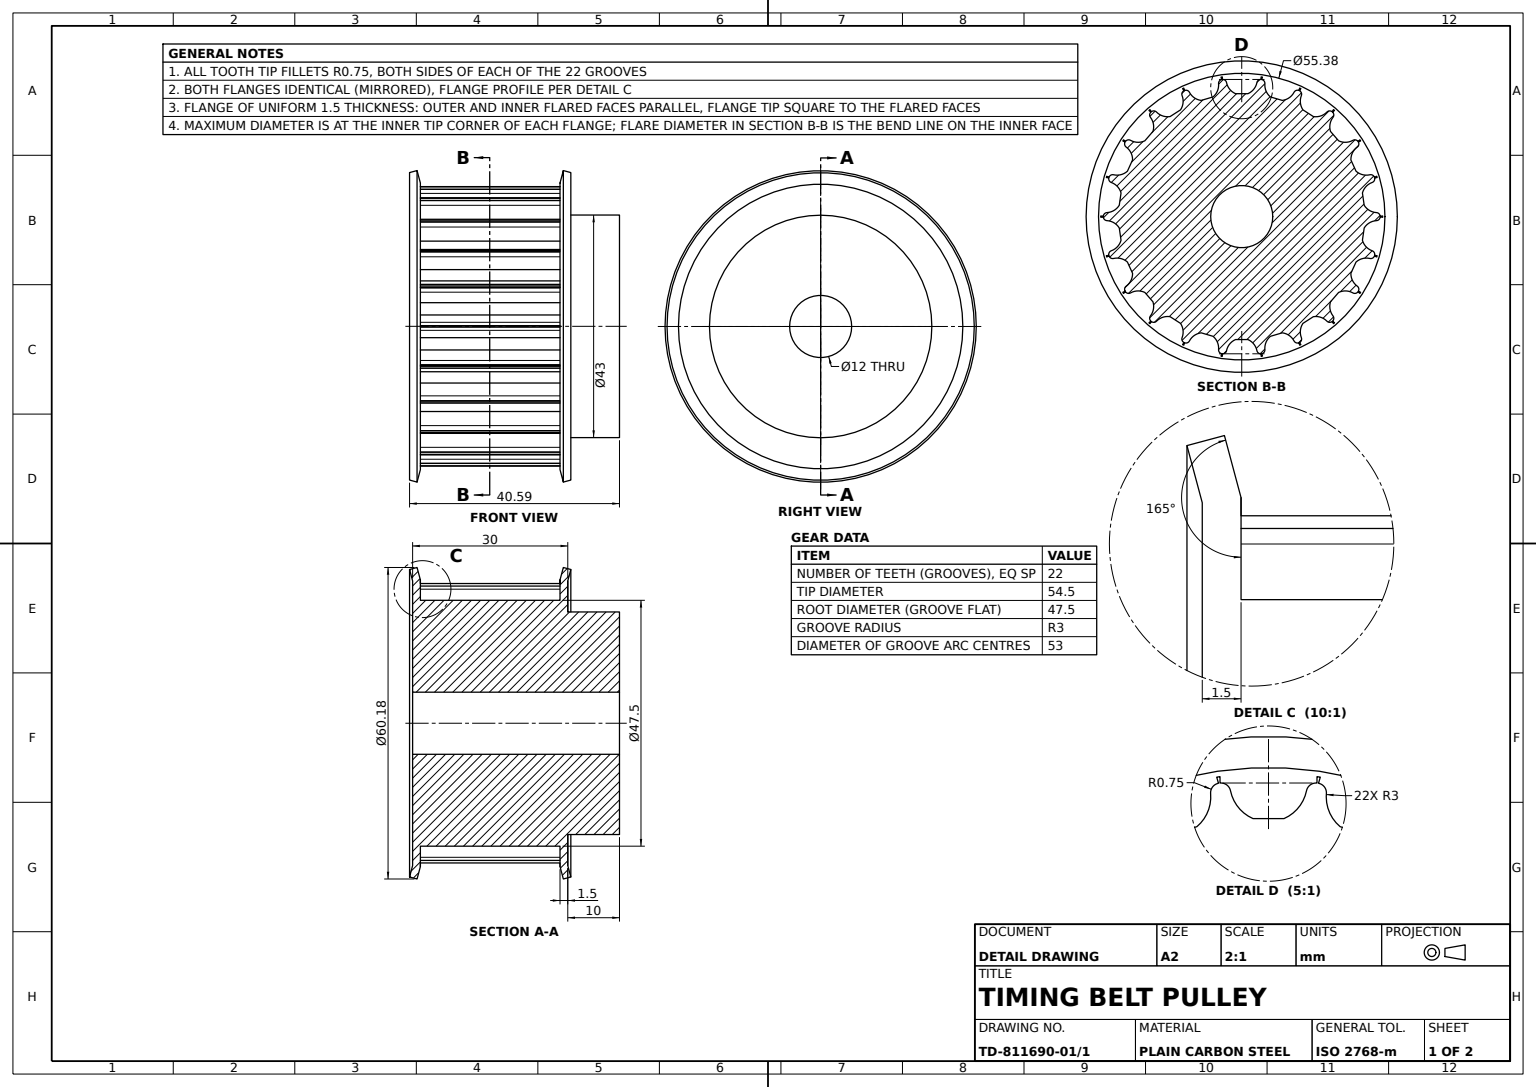
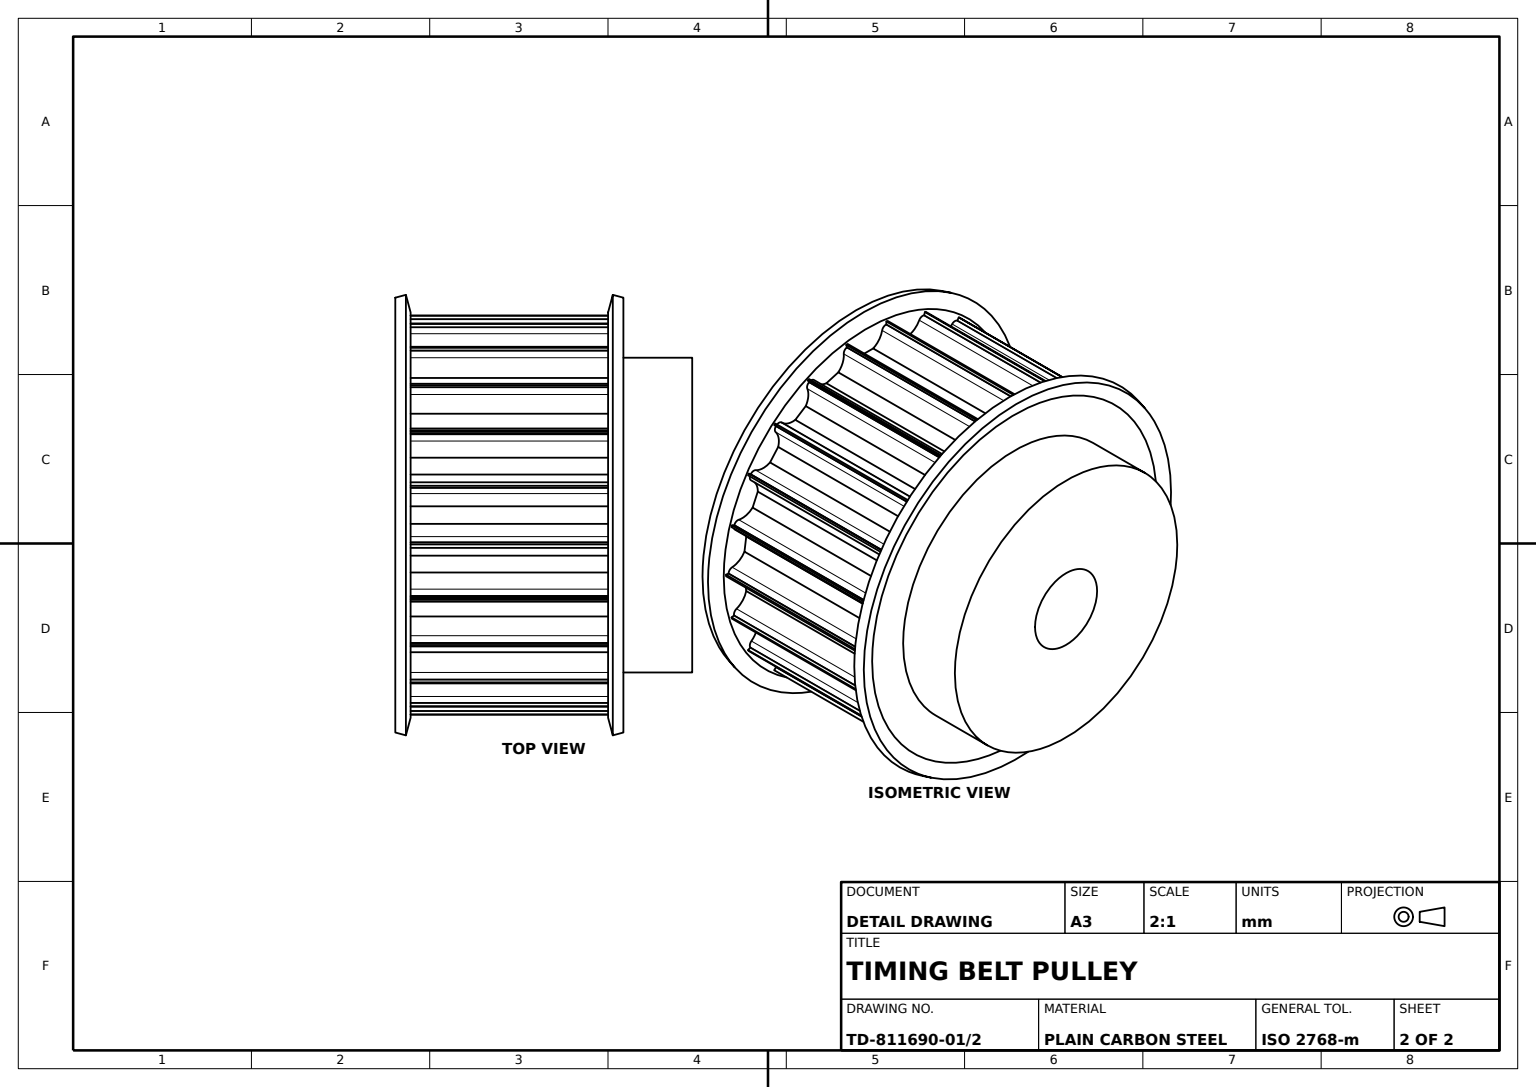
from build123d import *

# Parameters (mm, degrees)
TOOTH_GROOVE_CUT_DEPTH         = 56.543901555
TOOTH_GROOVE_PATTERN_22X_COUNT = 22


with BuildPart() as part:
    # Wheel Body Profile → Wheel Body (revolve)
    with BuildSketch(Plane(origin=(0, 0, 0), x_dir=(0, 0, -1), z_dir=(1, 0, 0)), mode=Mode.PRIVATE) as wheel_body_sk:
        Polygon((0, 6), (0, 27.25), (30, 27.25), (30, 21.5), (40, 21.5), (40, 6), align=None)
    revolve(wheel_body_sk.sketch.rotate(Axis((0, 0, -42.02959834), (0, 0, 1)), 90), axis=Axis((0, 0, -42.02959834), (0, 0, 1)))

    # Tooth Groove Profile → Tooth Groove Cut (cut, through all)
    with BuildSketch(Plane.XY):
        with BuildLine():
            Line((3.674234614, 26.5), (3.75, 26.5))
            Line((3.75, 26.5), (3.75, 28.5))
            Line((3.75, 28.5), (-3.75, 28.5))
            Line((-3.75, 28.5), (-3.75, 26.5))
            Line((-3.75, 26.5), (-3.674234614, 26.5))
            ThreePointArc((-3.674234614, 26.5), (-3.199892965, 26.330947502), (-2.939387691, 25.9))
            ThreePointArc((-2.939387691, 25.9), (-2.331759211, 24.612435701), (-1.198957881, 23.75))
            Line((-1.198957881, 23.75), (1.198957881, 23.75))
            ThreePointArc((1.198957881, 23.75), (2.331759211, 24.612435701), (2.939387691, 25.9))
            ThreePointArc((2.939387691, 25.9), (3.199892965, 26.330947502), (3.674234614, 26.5))
        make_face()
    tooth_groove_cut = extrude(amount=-TOOTH_GROOVE_CUT_DEPTH, mode=Mode.SUBTRACT)

    # Tooth Groove Pattern 22x: Tooth Groove Cut ×22 about axis
    tooth_groove_pattern_22x_axis = Axis((0, 0, 0), (0, 0, 1))
    for i in range(1, TOOTH_GROOVE_PATTERN_22X_COUNT):
        add(tooth_groove_cut.rotate(tooth_groove_pattern_22x_axis, i * 360 / TOOTH_GROOVE_PATTERN_22X_COUNT), mode=Mode.SUBTRACT)

    # Flange Profile → Belt Flanges (revolve)
    with BuildSketch(Plane(origin=(0, 0, 0), x_dir=(0, 0, -1), z_dir=(1, 0, 0)), mode=Mode.PRIVATE) as belt_flanges_sk:
        Polygon((0, 27.493260406), (0, 22.690739153), (1.5, 22.690739153), (1.5, 27.690739153), (0.856921938, 30.090739153), (-0.591966801, 29.702510585), align=None)
        Polygon((30.591966801, 29.702510585), (29.143078062, 30.090739153), (28.5, 27.690739153), (28.5, 22.690739153), (30, 22.690739153), (30, 27.493260406), align=None)
    revolve(belt_flanges_sk.sketch.rotate(Axis((0, 0, -42.02959834), (0, 0, 1)), 90), axis=Axis((0, 0, -42.02959834), (0, 0, 1)))


solid = part.part
